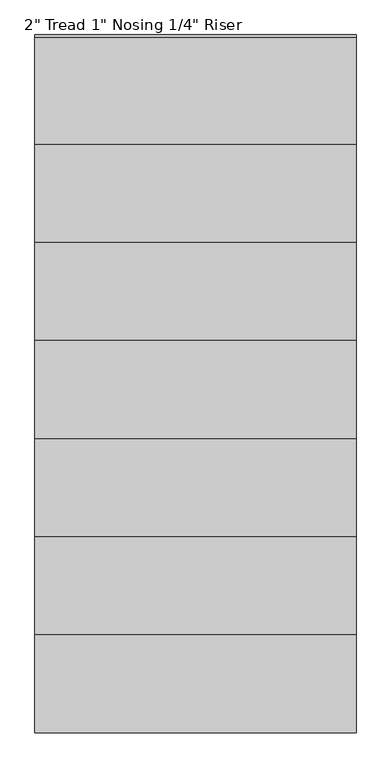
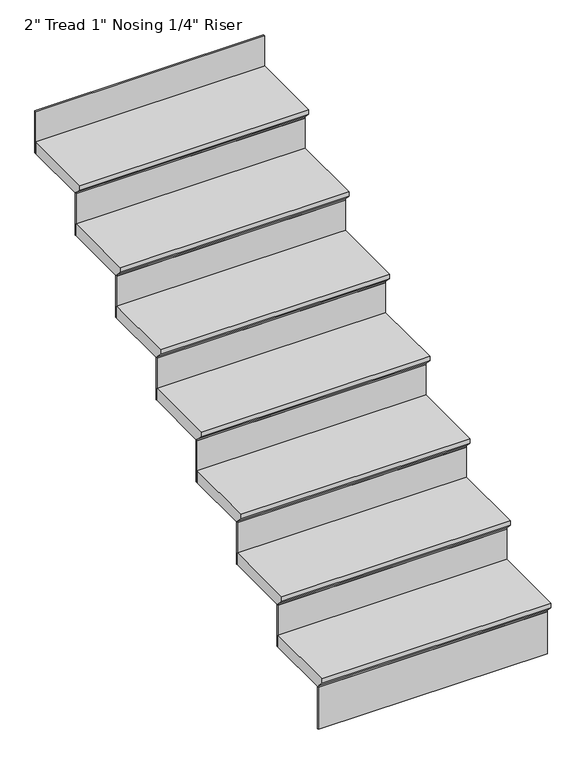
"""IFC4 building model written with IfcOpenShell, lengths in millimetres: stair flight geometry."""

from ifc_helpers import new_model, si_unit, frame, origin, place, context, project, spatial, polyline, outline, extrude, source, transform, mapped, element, save


def stair_flight_75ff7960(model_context):
    return source(origin(), model_context, "Body", "SweptSolid", [
        extrude(outline(polyline([(-3614.7064015, 2565.4), (-3309.9064015, 2565.4), (-3309.9064015, 2514.6), (-3589.3064015, 2514.6), (-3589.3064015, 2520.95), (-3614.7064015, 2546.35), (-3614.7064015, 2565.4)])), frame((13296.0761273, 0.0, 0.0), z_axis=(1.0, 0.0, 0.0), x_axis=(0.0, 1.0, 0.0)), (0.0, 0.0, 1.0), 914.4),
        extrude(outline(polyline([(14210.4761273, -3582.9564015), (14210.4761273, -3589.3064015), (13296.0761273, -3589.3064015), (13296.0761273, -3582.9564015), (14210.4761273, -3582.9564015)])), frame((0.0, 0.0, 2336.8), z_axis=(0.0, 0.0, 1.0), x_axis=(1.0, 0.0, 0.0)), (0.0, 0.0, 1.0), 177.8),
        extrude(outline(polyline([(14210.4761273, -3303.5564015), (14210.4761273, -3309.9064015), (13296.0761273, -3309.9064015), (13296.0761273, -3303.5564015), (14210.4761273, -3303.5564015)])), frame((0.0, 0.0, 2514.6), z_axis=(0.0, 0.0, 1.0), x_axis=(1.0, 0.0, 0.0)), (0.0, 0.0, 1.0), 177.8),
        extrude(outline(polyline([(-3335.3064015, 2743.2), (-3030.5064015, 2743.2), (-3030.5064015, 2692.4), (-3309.9064015, 2692.4), (-3309.9064015, 2698.75), (-3335.3064015, 2724.15), (-3335.3064015, 2743.2)])), frame((13296.0761273, 0.0, 0.0), z_axis=(1.0, 0.0, 0.0), x_axis=(0.0, 1.0, 0.0)), (0.0, 0.0, 1.0), 914.4),
        extrude(outline(polyline([(14210.4761273, -3024.1564015), (14210.4761273, -3030.5064015), (13296.0761273, -3030.5064015), (13296.0761273, -3024.1564015), (14210.4761273, -3024.1564015)])), frame((0.0, 0.0, 2692.4), z_axis=(0.0, 0.0, 1.0), x_axis=(1.0, 0.0, 0.0)), (0.0, 0.0, 1.0), 177.8),
        extrude(outline(polyline([(-3055.9064015, 2921.0), (-2751.1064015, 2921.0), (-2751.1064015, 2870.2), (-3030.5064015, 2870.2), (-3030.5064015, 2876.55), (-3055.9064015, 2901.95), (-3055.9064015, 2921.0)])), frame((13296.0761273, 0.0, 0.0), z_axis=(1.0, 0.0, 0.0), x_axis=(0.0, 1.0, 0.0)), (0.0, 0.0, 1.0), 914.4),
        extrude(outline(polyline([(14210.4761273, -2744.7564015), (14210.4761273, -2751.1064015), (13296.0761273, -2751.1064015), (13296.0761273, -2744.7564015), (14210.4761273, -2744.7564015)])), frame((0.0, 0.0, 2870.2), z_axis=(0.0, 0.0, 1.0), x_axis=(1.0, 0.0, 0.0)), (0.0, 0.0, 1.0), 177.8),
        extrude(outline(polyline([(-2776.5064015, 3098.8), (-2471.7064015, 3098.8), (-2471.7064015, 3048.0), (-2751.1064015, 3048.0), (-2751.1064015, 3054.35), (-2776.5064015, 3079.75), (-2776.5064015, 3098.8)])), frame((13296.0761273, 0.0, 0.0), z_axis=(1.0, 0.0, 0.0), x_axis=(0.0, 1.0, 0.0)), (0.0, 0.0, 1.0), 914.4),
        extrude(outline(polyline([(14210.4761273, -2465.3564015), (14210.4761273, -2471.7064015), (13296.0761273, -2471.7064015), (13296.0761273, -2465.3564015), (14210.4761273, -2465.3564015)])), frame((0.0, 0.0, 3048.0), z_axis=(0.0, 0.0, 1.0), x_axis=(1.0, 0.0, 0.0)), (0.0, 0.0, 1.0), 177.8),
        extrude(outline(polyline([(-2497.1064015, 3276.6), (-2192.3064015, 3276.6), (-2192.3064015, 3225.8), (-2471.7064015, 3225.8), (-2471.7064015, 3232.15), (-2497.1064015, 3257.55), (-2497.1064015, 3276.6)])), frame((13296.0761273, 0.0, 0.0), z_axis=(1.0, 0.0, 0.0), x_axis=(0.0, 1.0, 0.0)), (0.0, 0.0, 1.0), 914.4),
        extrude(outline(polyline([(14210.4761273, -2185.9564015), (14210.4761273, -2192.3064015), (13296.0761273, -2192.3064015), (13296.0761273, -2185.9564015), (14210.4761273, -2185.9564015)])), frame((0.0, 0.0, 3225.8), z_axis=(0.0, 0.0, 1.0), x_axis=(1.0, 0.0, 0.0)), (0.0, 0.0, 1.0), 177.8),
        extrude(outline(polyline([(-2217.7064015, 3454.4), (-1912.9064015, 3454.4), (-1912.9064015, 3403.6), (-2192.3064015, 3403.6), (-2192.3064015, 3409.95), (-2217.7064015, 3435.35), (-2217.7064015, 3454.4)])), frame((13296.0761273, 0.0, 0.0), z_axis=(1.0, 0.0, 0.0), x_axis=(0.0, 1.0, 0.0)), (0.0, 0.0, 1.0), 914.4),
        extrude(outline(polyline([(14210.4761273, -1906.5564015), (14210.4761273, -1912.9064015), (13296.0761273, -1912.9064015), (13296.0761273, -1906.5564015), (14210.4761273, -1906.5564015)])), frame((0.0, 0.0, 3403.6), z_axis=(0.0, 0.0, 1.0), x_axis=(1.0, 0.0, 0.0)), (0.0, 0.0, 1.0), 177.8),
        extrude(outline(polyline([(14210.4761273, -1627.1564015), (14210.4761273, -1633.5064015), (13296.0761273, -1633.5064015), (13296.0761273, -1627.1564015), (14210.4761273, -1627.1564015)])), frame((0.0, 0.0, 3581.4), z_axis=(0.0, 0.0, 1.0), x_axis=(1.0, 0.0, 0.0)), (0.0, 0.0, 1.0), 177.8),
        extrude(outline(polyline([(-1938.3064015, 3632.2), (-1633.5064015, 3632.2), (-1633.5064015, 3581.4), (-1912.9064015, 3581.4), (-1912.9064015, 3587.75), (-1938.3064015, 3613.15), (-1938.3064015, 3632.2)])), frame((13296.0761273, 0.0, 0.0), z_axis=(1.0, 0.0, 0.0), x_axis=(0.0, 1.0, 0.0)), (0.0, 0.0, 1.0), 914.4),
    ])


if __name__ == "__main__":
    model = new_model("IFC4")
    model_context = context("Model", 3, world=origin())
    ifc_project = project(units=[si_unit("LENGTHUNIT", "METRE", prefix="MILLI")], contexts=[model_context])
    site = spatial("IfcSite", under=ifc_project)
    building = spatial("IfcBuilding", under=site)
    placement = place(None, origin())
    stair_flight_shape = stair_flight_75ff7960(model_context)
    element("IfcStairFlight", 1, ObjectType="2\" Tread 1\" Nosing 1/4\" Riser", at=placement, inside=building, context=model_context, shape_type="MappedRepresentation", body=[
        mapped(stair_flight_shape, transform((0.0, 0.0, 0.0), x_axis=(1.0, 0.0, 0.0), y_axis=(0.0, 1.0, 0.0), z_axis=(0.0, 0.0, 1.0))),
    ])
    save(model, "model.ifc")
